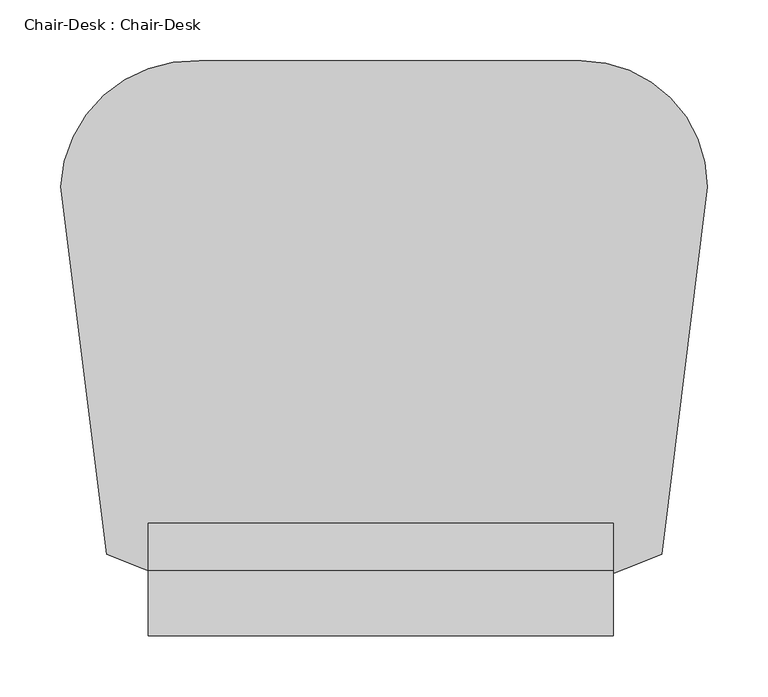
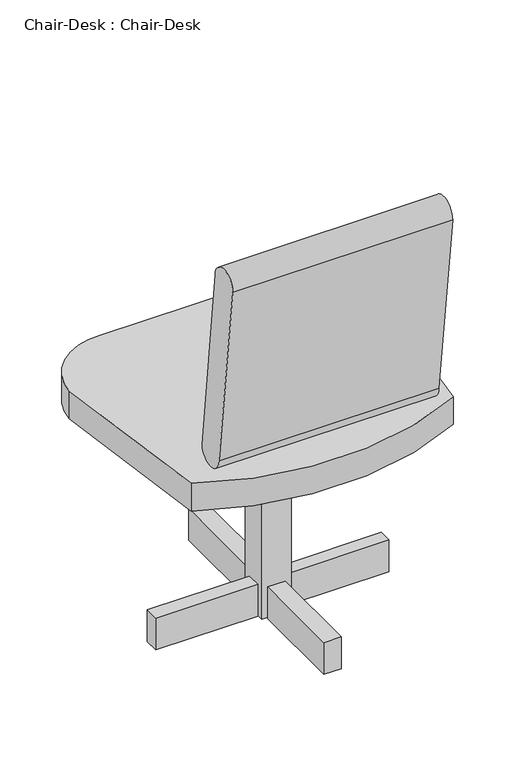
"""IFC4 building model written with IfcOpenShell, lengths in millimetres: furniture geometry, Chair-Desk : Chair-Desk."""

from ifc_helpers import new_model, si_unit, point, frame, frame_2d, origin, origin_with_axes, place, context, project, spatial, polyline, circle_curve, trimmed, segment, composite_curve, outline, extrude, source, transform, mapped, element, save


def chair_desk_chair_desk_ccc35c8f(model_context):
    return source(origin(), model_context, "Body", "SweptSolid", [
        extrude(outline(polyline([(-203.6618182, 175.0290909), (-25.8618182, 175.0290909), (-25.8618182, 150.0462968), (-203.6618182, 150.0462968), (-203.6618182, 175.0290909)])), origin_with_axes(), (0.0, 0.0, 1.0), 58.5040426),
        extrude(outline(polyline([(204.1236364, 175.0290909), (204.1236364, 152.4), (26.7854545, 152.4), (26.7854545, 175.0290909), (204.1236364, 175.0290909)])), origin_with_axes(), (0.0, 0.0, 1.0), 58.5040426),
        extrude(outline(polyline([(-16.1636364, 188.8836364), (-16.1636364, 374.9517514), (14.3163636, 374.9517514), (14.3163636, 188.8836364), (-16.1636364, 188.8836364)])), origin_with_axes(), (0.0, 0.0, 1.0), 58.5040426),
        extrude(outline(polyline([(14.3163636, 136.2363636), (14.3163636, -33.2509091), (-16.1636364, -33.2509091), (-16.1636364, 136.2363636), (14.3163636, 136.2363636)])), origin_with_axes(), (0.0, 0.0, 1.0), 58.5040426),
        extrude(outline(polyline([(26.3236364, 190.2690909), (26.3236364, 139.4690909), (-24.4763636, 139.4690909), (-24.4763636, 190.2690909), (26.3236364, 190.2690909)])), origin_with_axes(), (0.0, 0.0, 1.0), 355.6),
        extrude(outline(composite_curve([segment(polyline([(-13.6321252, 787.4), (25.5523927, 451.3880753)]), True, "CONTINUOUS"), segment(trimmed(circle_curve(frame_2d((0.0761963, 451.3880753)), 25.4761963), [point((25.5523927, 451.3880753))], [point((-25.4, 451.3880753))], False, "CARTESIAN"), True, "CONTINUOUS"), segment(polyline([(-25.4, 451.3880753), (-67.209111, 787.4)]), True, "CONTINUOUS"), segment(trimmed(circle_curve(frame_2d((-40.4206181, 787.4)), 26.7884929), [point((-67.209111, 787.4))], [point((-13.6321252, 787.4))], False, "CARTESIAN"), True, "CONTINUOUS")], self_intersect=False)), frame((-194.3643056, 0.0, 0.0), z_axis=(1.0, 0.0, 0.0), x_axis=(0.0, 1.0, 0.0)), (0.0, 0.0, 1.0), 383.2768056),
        extrude(outline(composite_curve([segment(trimmed(circle_curve(frame_2d((-157.1362322, 297.1024212)), 109.4001491), [point((-266.4057871, 302.4462968))], [point((-152.4, 406.4))], False, "CARTESIAN"), True, "CONTINUOUS"), segment(polyline([(-152.4, 406.4), (162.2530084, 406.4)]), True, "CONTINUOUS"), segment(trimmed(circle_curve(frame_2d((162.2530084, 302.4462968)), 103.9537032), [point((162.2530084, 406.4))], [point((266.2067116, 302.4462968))], False, "CARTESIAN"), True, "CONTINUOUS"), segment(polyline([(266.2067116, 302.4462968), (228.6, 0.0)]), True, "CONTINUOUS"), segment(trimmed(circle_curve(frame_2d((0.0, 446.8941036)), 501.9684252), [point((228.6, 0.0))], [point((-228.6, 0.0))], False, "CARTESIAN"), True, "CONTINUOUS"), segment(polyline([(-228.6, 0.0), (-266.4057871, 302.4462968)]), True, "CONTINUOUS")], self_intersect=False)), frame((0.0, 0.0, 355.6), z_axis=(0.0, 0.0, 1.0), x_axis=(1.0, 0.0, 0.0)), (0.0, 0.0, 1.0), 50.8),
    ])


if __name__ == "__main__":
    model = new_model("IFC4")
    model_context = context("Model", 3, world=origin())
    ifc_project = project(units=[si_unit("LENGTHUNIT", "METRE", prefix="MILLI")], contexts=[model_context])
    site = spatial("IfcSite", under=ifc_project)
    building = spatial("IfcBuilding", under=site)
    placement = place(None, origin())
    chair_desk_chair_desk_shape = chair_desk_chair_desk_ccc35c8f(model_context)
    element("IfcFurniture", 1, ObjectType="Chair-Desk : Chair-Desk", at=placement, inside=building, context=model_context, shape_type="MappedRepresentation", body=[
        mapped(chair_desk_chair_desk_shape, transform((0.0, 0.0, 0.0), x_axis=(1.0, 0.0, 0.0), y_axis=(0.0, 1.0, 0.0), z_axis=(0.0, 0.0, 1.0))),
    ])
    save(model, "model.ifc")

# Revit data of these elements
# Type "Chair-Desk : Chair-Desk"
#   Assembly Code = "E2020200"
#   Seat/Back Material = Textile - Slate Blue
#   Base Material = Steel, Chrome Plated
#   Default Elevation = 0
# Element 1 (IfcFurniture, "Chair-Desk : Chair-Desk")
#   Materials on its faces: "Steel, Chrome Plated", "Textile - Slate Blue"
# Materials
#   "Textile - Slate Blue": class "Fabric", colour RGB 98 102 118, transparency 0
#   "Steel, Chrome Plated": class "Metal", colour RGB 17 17 17, transparency 0, Description = "Chromiuim plated steel", Cost = 0
